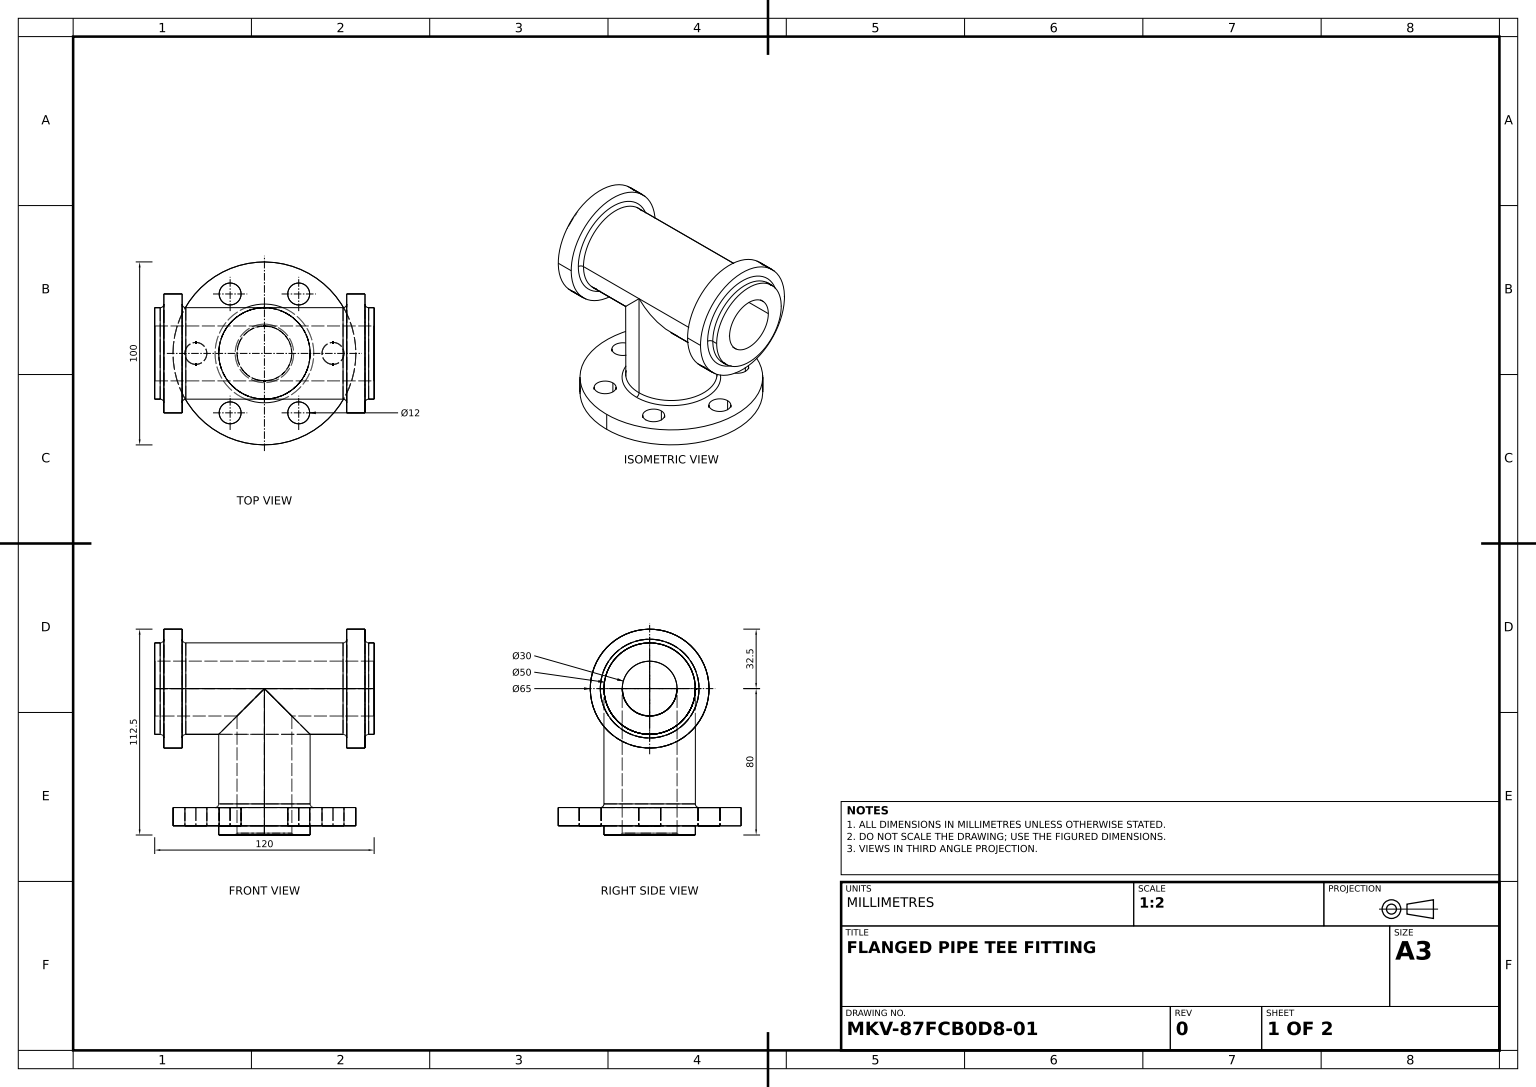
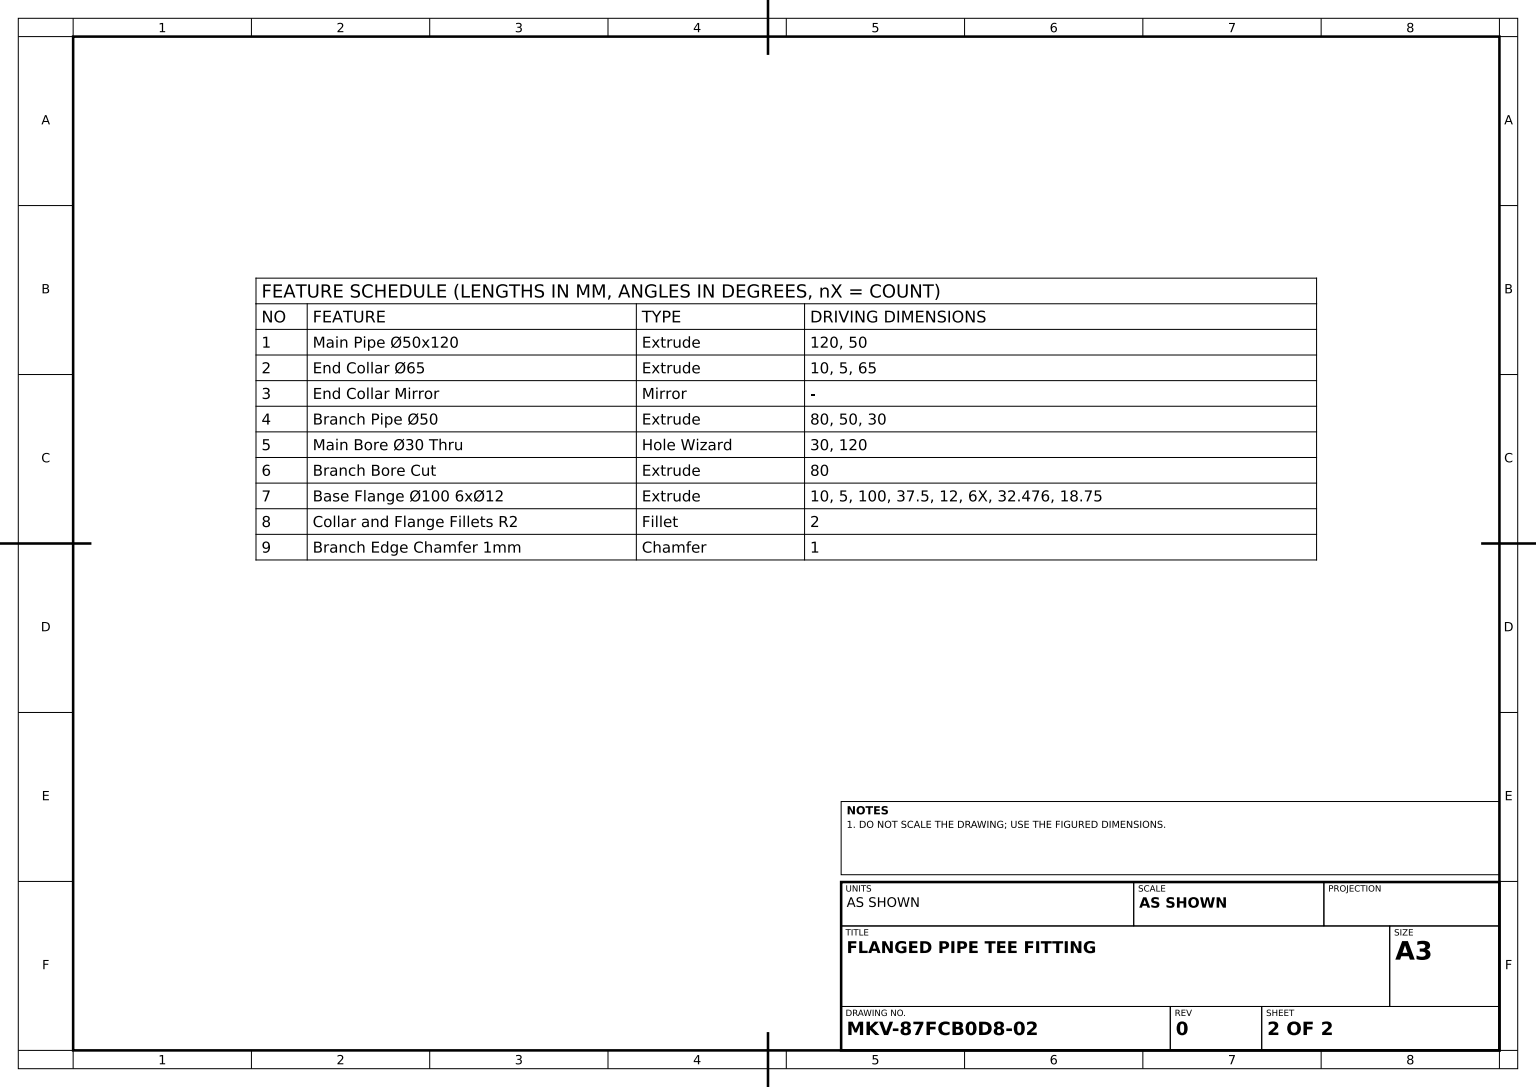
from build123d import *

# Parameters (mm, degrees)
MAIN_PIPE_SKETCH_R             = 25
MAIN_PIPE_50X120_DEPTH         = 60
END_START                      = -5
END_COLLAR_SKETCH_R            = 32.5
END_COLLAR_SKETCH_R_2          = 25
END_COLLAR_65_DEPTH            = 10
BRANCH_PIPE_SKETCH_R           = 25
BRANCH_PIPE_SKETCH_R_2         = 15
BRANCH_PIPE_50_DEPTH           = 80
MAIN_BORE_30_THRU_D            = 30
BRANCH_BORE_SKETCH_R           = 15
BRANCH_BORE_CUT_DEPTH          = 80
BASE_START                     = -15
BASE_FLANGE_SKETCH_R           = 50
BASE_FLANGE_SKETCH_R_2         = 6
BASE_FLANGE_SKETCH_R_3         = 25
BASE_FLANGE_100_6X_12_DEPTH    = 10
COLLAR_AND_FLANGE_FILLETS_R2_R = 2
BRANCH_EDGE_CHAMFER_1MM_SIZE   = 1


with BuildPart() as part:
    # Main Pipe Sketch → Main Pipe Ø50x120 (new, symmetric)
    with BuildSketch(Plane(origin=(0, 0, 0), x_dir=(0, 0, -1), z_dir=(1, 0, 0))):
        Circle(MAIN_PIPE_SKETCH_R)
    extrude(amount=MAIN_PIPE_50X120_DEPTH, both=True)

    # End Collar Sketch → End Collar Ø65 (add)
    with BuildSketch(Plane(origin=(60, 0, 0), x_dir=(0, 0, -1), z_dir=(1, 0, 0)).offset(END_START)):
        Circle(END_COLLAR_SKETCH_R)
        Circle(END_COLLAR_SKETCH_R_2, mode=Mode.SUBTRACT)
    end_collar_65 = extrude(amount=-END_COLLAR_65_DEPTH)

    # End Collar Mirror: End Collar Ø65 across plane
    add(end_collar_65.mirror(Plane(origin=(0, 0, 0), x_dir=(0, 0, 1), z_dir=(1, 0, 0))))

    # Branch Pipe Sketch → Branch Pipe Ø50 (add)
    with BuildSketch(Plane(origin=(0, 0, 0), x_dir=(1, 0, 0), z_dir=(0, 1, 0))):
        with Locations(Location((0, 0, 0), (0, 0, 270))):
            Circle(BRANCH_PIPE_SKETCH_R)
        with Locations(Location((0, 0, 0), (0, 0, 270))):
            Circle(BRANCH_PIPE_SKETCH_R_2, mode=Mode.SUBTRACT)
    extrude(amount=-BRANCH_PIPE_50_DEPTH)

    # Main Bore Ø30 Thru (through all)
    with Locations(Plane(origin=(60, 0, 0), x_dir=(0, 0, -1), z_dir=(1, 0, 0))):
        with Locations((0, 0)):
            Hole(MAIN_BORE_30_THRU_D / 2)

    # Branch Bore Sketch → Branch Bore Cut (cut)
    with BuildSketch(Plane(origin=(0, 0, 0), x_dir=(1, 0, 0), z_dir=(0, 1, 0))):
        with Locations(Location((0, 0, 0), (0, 0, 270))):
            Circle(BRANCH_BORE_SKETCH_R)
    extrude(amount=-BRANCH_BORE_CUT_DEPTH, mode=Mode.SUBTRACT)

    # Base Flange Sketch → Base Flange Ø100 6xØ12 (add)
    with BuildSketch(Plane.XZ.offset(80).offset(BASE_START)):
        with Locations(Location((0, 0, 0), (0, 0, 270))):
            Circle(BASE_FLANGE_SKETCH_R)
        with Locations(Location((37.5, 0, 0), (0, 0, 270))):
            Circle(BASE_FLANGE_SKETCH_R_2, mode=Mode.SUBTRACT)
        with Locations(Location((0, 0, 0), (0, 0, 270))):
            Circle(BASE_FLANGE_SKETCH_R_3, mode=Mode.SUBTRACT)
        with Locations(Location((18.75, -32.475952642, 0), (0, 0, 270))):
            Circle(BASE_FLANGE_SKETCH_R_2, mode=Mode.SUBTRACT)
        with Locations(Location((-18.75, -32.475952642, 0), (0, 0, 270))):
            Circle(BASE_FLANGE_SKETCH_R_2, mode=Mode.SUBTRACT)
        with Locations(Location((-37.5, 0, 0), (0, 0, 270))):
            Circle(BASE_FLANGE_SKETCH_R_2, mode=Mode.SUBTRACT)
        with Locations(Location((-18.75, 32.475952642, 0), (0, 0, 270))):
            Circle(BASE_FLANGE_SKETCH_R_2, mode=Mode.SUBTRACT)
        with Locations(Location((18.75, 32.475952642, 0), (0, 0, 270))):
            Circle(BASE_FLANGE_SKETCH_R_2, mode=Mode.SUBTRACT)
    extrude(amount=BASE_FLANGE_100_6X_12_DEPTH)

    # Collar and Flange Fillets R2
    collar_and_flange_fillets_r2_edges = [part.edges().sort_by_distance(p)[0] for p in [
        (-45, 0, 25),
        (-55, 0, 25),
        (0, -65, -25),
        (45, 0, 25),
        (55, 0, 25),
    ]]
    fillet(collar_and_flange_fillets_r2_edges, radius=COLLAR_AND_FLANGE_FILLETS_R2_R)

    # Branch Edge Chamfer 1mm
    branch_edge_chamfer_1mm_edges = [part.edges().sort_by_distance(p)[0] for p in [
        (0, -80, -15),
    ]]
    chamfer(branch_edge_chamfer_1mm_edges, length=BRANCH_EDGE_CHAMFER_1MM_SIZE)


solid = part.part
